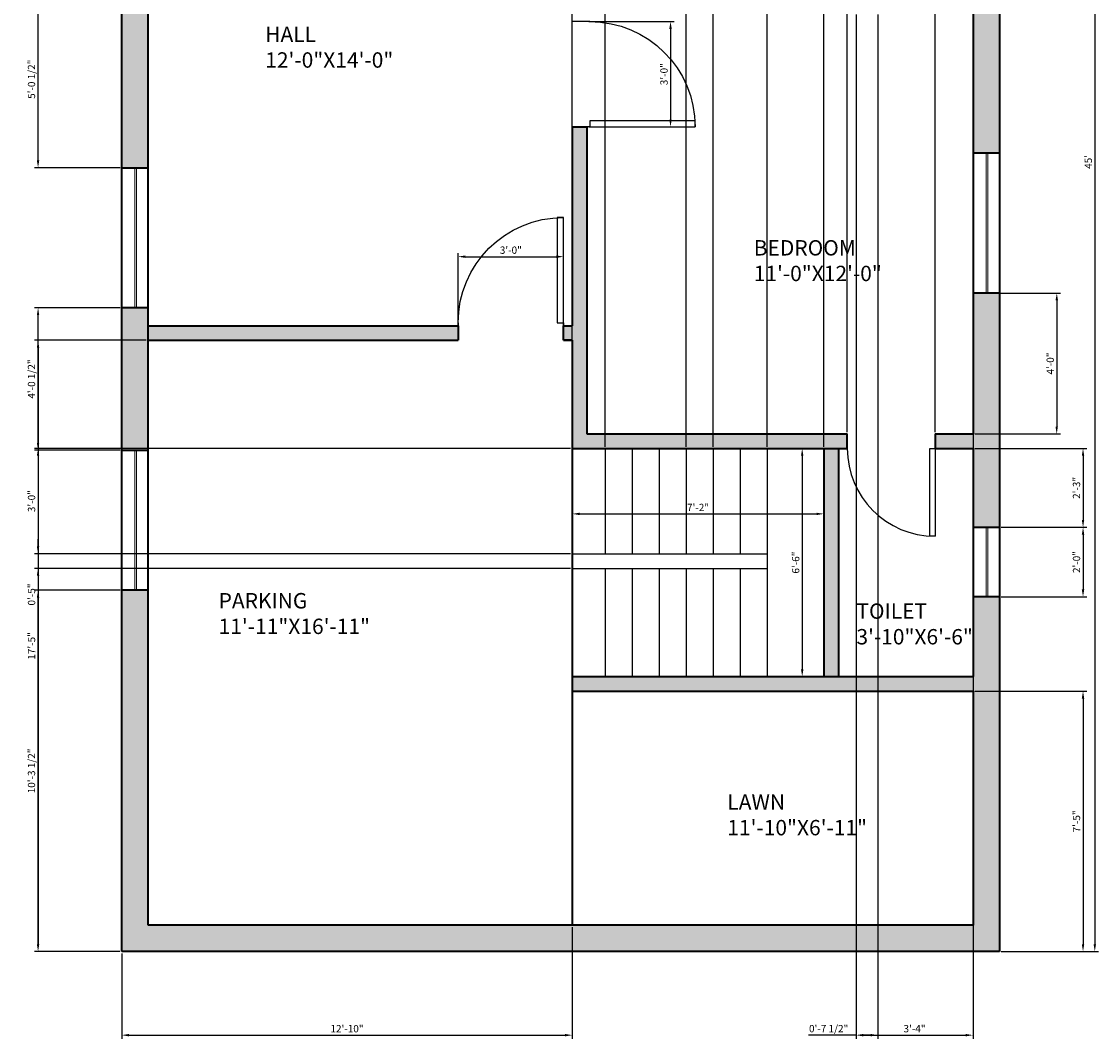
# Model space of a CAD drawing. Units: inches. Extents: x 2545 to 2915, y 1754 to 2359.
# Tile 1 of 2: x 2545 to 2913, y 1754 to 2103. Entities that reach past the tile are written whole.
import ezdxf

# ---------------------------------------------------------------- set-up
doc = ezdxf.new("R2010")
doc.units = ezdxf.units.IN
for name, color, linetype, lineweight in [('A-ANNO-DIMS', 2, 'Continuous', 18), ('A-AREA-IDEN', 7, 'Continuous', 25), ('A-DOOR', 3, 'Continuous', 25), ('A-FLOR-STRS', 7, 'Continuous', 25), ('A-GLAZ', 4, 'Continuous', 18), ('A-WALL', 7, 'Continuous', 35), ('A-WALL-PATT', 252, 'Continuous', 13)]:
    doc.layers.add(name, color=color, linetype=linetype, lineweight=lineweight)
doc.styles.get("Standard").update_dxf_attribs({"font": 'arial.ttf'})
doc.dimstyles.new('ISO-25', dxfattribs={"dimtxt": 2.5, "dimasz": 2.5, "dimexe": 1.25, "dimexo": 0.625, "dimtad": 1, "dimlunit": 4, "dimtxsty": 'Standard', "dimcen": 2.5, "dimadec": 0, "dimazin": 0, "dimtfac": 1, "dimtmove": 0, "dimatfit": 3, "dimfxl": 1, "dimarcsym": 0})

# ---------------------------------------------------------------- blocks, each defined once
blk = doc.blocks.new('*U2')
for p, q in [((0, 0), (0, -5)), ((30, 0), (30, -5))]:
    blk.add_line(p, q)
blk.add_lwpolyline([(0, 0), (0, 30), (1.75, 30), (1.75, 0)], close=True)
blk.add_arc((0, 0), 30, 0, 90)
blk = doc.blocks.new('*D4')
at = {"layer": 'A-ANNO-DIMS', "color": 0, "lineweight": -2, "transparency": 16777216}
for p, q in [((2880.02, 2324.74), (2913.27, 2324.74)), ((2912.02, 2322.24), (2912.02, 1787.24)), ((2880.02, 1784.74), (2913.27, 1784.74))]:
    blk.add_line(p, q, dxfattribs=at)
at = {"layer": 'A-ANNO-DIMS', "color": 0, "transparency": 16777216}
for points in [[(2911.6, 2322.24), (2912.44, 2322.24), (2912.02, 2324.74)], [(2911.6, 1787.24), (2912.44, 1787.24), (2912.02, 1784.74)]]:
    blk.add_solid(points, dxfattribs=at)
at = {"layer": 'Defpoints', "color": 0, "transparency": 16777216}
for p in [(2879.4, 2324.74), (2879.4, 1784.74), (2912.02, 1784.74)]:
    blk.add_point(p, dxfattribs=at)
at = {"layer": 'A-ANNO-DIMS', "color": 0, "transparency": 16777216, "insert": (2910.12, 2054.74), "char_height": 2.5, "attachment_point": 5, "rotation": 90}
blk.add_mtext("45'", dxfattribs=at)
blk = doc.blocks.new('*D5')
at = {"layer": 'A-ANNO-DIMS', "color": 0, "lineweight": -2, "transparency": 16777216}
for p, q in [((2809.58, 1956.74), (2813.25, 1956.74)), ((2812, 1954.24), (2812, 1881.24)), ((2809.58, 1878.74), (2813.25, 1878.74))]:
    blk.add_line(p, q, dxfattribs=at)
at = {"layer": 'A-ANNO-DIMS', "color": 0, "transparency": 16777216}
for points in [[(2811.59, 1954.24), (2812.42, 1954.24), (2812, 1956.74)], [(2811.59, 1881.24), (2812.42, 1881.24), (2812, 1878.74)]]:
    blk.add_solid(points, dxfattribs=at)
at = {"layer": 'Defpoints', "color": 0, "transparency": 16777216}
for p in [(2808.96, 1956.74), (2808.96, 1878.74), (2812, 1878.74)]:
    blk.add_point(p, dxfattribs=at)
at = {"layer": 'A-ANNO-DIMS', "color": 0, "transparency": 16777216, "insert": (2810.1, 1917.74), "char_height": 2.5, "attachment_point": 5, "rotation": 90}
blk.add_mtext('6\'-6"', dxfattribs=at)
blk = doc.blocks.new('*D6')
at = {"layer": 'A-ANNO-DIMS', "color": 0, "lineweight": -2, "transparency": 16777216}
for p, q in [((2733.4, 1931.78), (2733.4, 1935.64)), ((2735.9, 1934.39), (2816.9, 1934.39)), ((2819.4, 1931.78), (2819.4, 1935.64))]:
    blk.add_line(p, q, dxfattribs=at)
at = {"layer": 'A-ANNO-DIMS', "color": 0, "transparency": 16777216}
for points in [[(2735.9, 1934.8), (2735.9, 1933.97), (2733.4, 1934.39)], [(2816.9, 1934.8), (2816.9, 1933.97), (2819.4, 1934.39)]]:
    blk.add_solid(points, dxfattribs=at)
at = {"layer": 'Defpoints', "color": 0, "transparency": 16777216}
for p in [(2819.4, 1934.39), (2733.4, 1931.15), (2819.4, 1931.15)]:
    blk.add_point(p, dxfattribs=at)
at = {"layer": 'A-ANNO-DIMS', "color": 0, "transparency": 16777216, "insert": (2776.4, 1936.27), "char_height": 2.5, "attachment_point": 5}
blk.add_mtext('7\'-2"', dxfattribs=at)
blk = doc.blocks.new('WIN-SASH-48')
for p, q in [((0, 8.97), (47.9, 8.97)), ((0, 4.48), (47.9, 4.48)), ((0, 3.98), (47.9, 3.98)), ((47.9, 0), (0, 0))]:
    blk.add_line(p, q)
blk = doc.blocks.new('*D13')
at = {"layer": 'A-ANNO-DIMS', "color": 0, "lineweight": -2, "transparency": 16777216}
for p, q in [((2578.81, 1908.27), (2549.55, 1908.27)), ((2550.8, 1787.24), (2550.8, 1905.77)), ((2578.77, 1784.74), (2549.55, 1784.74))]:
    blk.add_line(p, q, dxfattribs=at)
at = {"layer": 'A-ANNO-DIMS', "color": 0, "transparency": 16777216}
for points in [[(2550.38, 1905.77), (2551.21, 1905.77), (2550.8, 1908.27)], [(2550.38, 1787.24), (2551.21, 1787.24), (2550.8, 1784.74)]]:
    blk.add_solid(points, dxfattribs=at)
at = {"layer": 'Defpoints', "color": 0, "transparency": 16777216}
for p in [(2550.8, 1908.27), (2579.43, 1908.27), (2579.4, 1784.74)]:
    blk.add_point(p, dxfattribs=at)
at = {"layer": 'A-ANNO-DIMS', "color": 0, "transparency": 16777216, "insert": (2548.88, 1846.5), "char_height": 2.5, "attachment_point": 5, "rotation": 90}
blk.add_mtext('10\'-3 1/2"', dxfattribs=at)
blk = doc.blocks.new('*D14')
at = {"layer": 'A-ANNO-DIMS', "color": 0, "lineweight": -2, "transparency": 16777216}
for p, q in [((2578.81, 2004.84), (2549.55, 2004.84)), ((2550.8, 1958.67), (2550.8, 2002.34)), ((2578.81, 1956.17), (2549.55, 1956.17))]:
    blk.add_line(p, q, dxfattribs=at)
at = {"layer": 'A-ANNO-DIMS', "color": 0, "transparency": 16777216}
for points in [[(2550.38, 2002.34), (2551.21, 2002.34), (2550.8, 2004.84)], [(2550.38, 1958.67), (2551.21, 1958.67), (2550.8, 1956.17)]]:
    blk.add_solid(points, dxfattribs=at)
at = {"layer": 'Defpoints', "color": 0, "transparency": 16777216}
for p in [(2550.8, 2004.84), (2579.43, 2004.84), (2579.43, 1956.17)]:
    blk.add_point(p, dxfattribs=at)
at = {"layer": 'A-ANNO-DIMS', "color": 0, "transparency": 16777216, "insert": (2548.88, 1980.5), "char_height": 2.5, "attachment_point": 5, "rotation": 90}
blk.add_mtext('4\'-0 1/2"', dxfattribs=at)
blk = doc.blocks.new('*D15')
at = {"layer": 'A-ANNO-DIMS', "color": 0, "lineweight": -2, "transparency": 16777216}
for p, q in [((2578.81, 2113.29), (2549.55, 2113.29)), ((2550.8, 2055.24), (2550.8, 2110.79)), ((2578.81, 2052.74), (2549.55, 2052.74))]:
    blk.add_line(p, q, dxfattribs=at)
at = {"layer": 'A-ANNO-DIMS', "color": 0, "transparency": 16777216}
for points in [[(2550.38, 2110.79), (2551.21, 2110.79), (2550.8, 2113.29)], [(2550.38, 2055.24), (2551.21, 2055.24), (2550.8, 2052.74)]]:
    blk.add_solid(points, dxfattribs=at)
at = {"layer": 'Defpoints', "color": 0, "transparency": 16777216}
for p in [(2550.8, 2113.29), (2579.43, 2113.29), (2579.43, 2052.74)]:
    blk.add_point(p, dxfattribs=at)
at = {"layer": 'A-ANNO-DIMS', "color": 0, "transparency": 16777216, "insert": (2548.88, 2083.01), "char_height": 2.5, "attachment_point": 5, "rotation": 90}
blk.add_mtext('5\'-0 1/2"', dxfattribs=at)
blk = doc.blocks.new('*D18')
at = {"layer": 'A-ANNO-DIMS', "color": 0, "lineweight": -2, "transparency": 16777216}
for p, q in [((2871.06, 2009.91), (2900.28, 2009.88)), ((2899.03, 2007.39), (2899, 1964.22)), ((2871.02, 1961.74), (2900.25, 1961.72))]:
    blk.add_line(p, q, dxfattribs=at)
at = {"layer": 'A-ANNO-DIMS', "color": 0, "transparency": 16777216}
for points in [[(2898.61, 2007.39), (2899.45, 2007.39), (2899.03, 2009.89)], [(2898.58, 1964.22), (2899.41, 1964.22), (2899, 1961.72)]]:
    blk.add_solid(points, dxfattribs=at)
at = {"layer": 'Defpoints', "color": 0, "transparency": 16777216}
for p in [(2870.43, 2009.91), (2870.4, 1961.74), (2899, 1961.72)]:
    blk.add_point(p, dxfattribs=at)
at = {"layer": 'A-ANNO-DIMS', "color": 0, "transparency": 16777216, "insert": (2897.11, 1985.8), "char_height": 2.5, "attachment_point": 5, "rotation": 89.9593}
blk.add_mtext('4\'-0"', dxfattribs=at)
blk = doc.blocks.new('*D21')
at = {"layer": 'A-ANNO-DIMS', "color": 0, "lineweight": -2, "transparency": 16777216}
for p, q in [((2694.4, 1994.37), (2694.4, 2023.59)), ((2696.9, 2022.34), (2727.9, 2022.34)), ((2730.4, 1994.37), (2730.4, 2023.59))]:
    blk.add_line(p, q, dxfattribs=at)
at = {"layer": 'A-ANNO-DIMS', "color": 0, "transparency": 16777216}
for points in [[(2696.9, 2022.76), (2696.9, 2021.92), (2694.4, 2022.34)], [(2727.9, 2022.76), (2727.9, 2021.92), (2730.4, 2022.34)]]:
    blk.add_solid(points, dxfattribs=at)
at = {"layer": 'Defpoints', "color": 0, "transparency": 16777216}
for p in [(2730.4, 2022.34), (2694.4, 1993.74), (2730.4, 1993.74)]:
    blk.add_point(p, dxfattribs=at)
at = {"layer": 'A-ANNO-DIMS', "color": 0, "transparency": 16777216, "insert": (2712.4, 2024.24), "char_height": 2.5, "attachment_point": 5}
blk.add_mtext('3\'-0"', dxfattribs=at)
blk = doc.blocks.new('*D24')
at = {"layer": 'A-ANNO-DIMS', "color": 0, "lineweight": -2, "transparency": 16777216}
for p, q in [((2739.02, 2102.74), (2768.25, 2102.74)), ((2767, 2100.24), (2767, 2069.24)), ((2739.02, 2066.74), (2768.25, 2066.74))]:
    blk.add_line(p, q, dxfattribs=at)
at = {"layer": 'A-ANNO-DIMS', "color": 0, "transparency": 16777216}
for points in [[(2766.58, 2100.24), (2767.41, 2100.24), (2767, 2102.74)], [(2766.58, 2069.24), (2767.41, 2069.24), (2767, 2066.74)]]:
    blk.add_solid(points, dxfattribs=at)
at = {"layer": 'Defpoints', "color": 0, "transparency": 16777216}
for p in [(2738.4, 2102.74), (2738.4, 2066.74), (2767, 2066.74)]:
    blk.add_point(p, dxfattribs=at)
at = {"layer": 'A-ANNO-DIMS', "color": 0, "transparency": 16777216, "insert": (2765.09, 2084.74), "char_height": 2.5, "attachment_point": 5, "rotation": 90}
blk.add_mtext('3\'-0"', dxfattribs=at)
blk = doc.blocks.new('*D26')
at = {"layer": 'A-ANNO-DIMS', "color": 0, "lineweight": -2, "transparency": 16777216}
for p, q in [((2733.4, 1793.12), (2733.4, 1754.89)), ((2579.4, 1784.12), (2579.4, 1754.89)), ((2581.9, 1756.14), (2730.9, 1756.14))]:
    blk.add_line(p, q, dxfattribs=at)
at = {"layer": 'A-ANNO-DIMS', "color": 0, "transparency": 16777216}
for points in [[(2581.9, 1756.56), (2581.9, 1755.72), (2579.4, 1756.14)], [(2730.9, 1756.56), (2730.9, 1755.72), (2733.4, 1756.14)]]:
    blk.add_solid(points, dxfattribs=at)
at = {"layer": 'Defpoints', "color": 0, "transparency": 16777216}
for p in [(2733.4, 1793.74), (2579.4, 1784.74), (2733.4, 1756.14)]:
    blk.add_point(p, dxfattribs=at)
at = {"layer": 'A-ANNO-DIMS', "color": 0, "transparency": 16777216, "insert": (2656.4, 1758.04), "char_height": 2.5, "attachment_point": 5}
blk.add_mtext('12\'-10"', dxfattribs=at)
blk = doc.blocks.new('*D27')
at = {"layer": 'A-ANNO-DIMS', "color": 0, "lineweight": -2, "transparency": 16777216}
for p, q in [((2587.77, 1993.74), (2549.55, 1993.74)), ((2550.8, 1991.24), (2550.8, 1787.24)), ((2578.77, 1784.74), (2549.55, 1784.74))]:
    blk.add_line(p, q, dxfattribs=at)
at = {"layer": 'A-ANNO-DIMS', "color": 0, "transparency": 16777216}
for points in [[(2550.38, 1991.24), (2551.21, 1991.24), (2550.8, 1993.74)], [(2550.38, 1787.24), (2551.21, 1787.24), (2550.8, 1784.74)]]:
    blk.add_solid(points, dxfattribs=at)
at = {"layer": 'Defpoints', "color": 0, "transparency": 16777216}
for p in [(2588.4, 1993.74), (2550.8, 1784.74), (2579.4, 1784.74)]:
    blk.add_point(p, dxfattribs=at)
at = {"layer": 'A-ANNO-DIMS', "color": 0, "transparency": 16777216, "insert": (2548.89, 1889.24), "char_height": 2.5, "attachment_point": 5, "rotation": 90}
blk.add_mtext('17\'-5"', dxfattribs=at)
blk = doc.blocks.new('*D28')
at = {"layer": 'A-ANNO-DIMS', "color": 0, "lineweight": -2, "transparency": 16777216}
for p, q in [((2871.02, 1873.74), (2909.25, 1873.74)), ((2908, 1871.24), (2908, 1787.24)), ((2880.02, 1784.74), (2909.25, 1784.74))]:
    blk.add_line(p, q, dxfattribs=at)
at = {"layer": 'A-ANNO-DIMS', "color": 0, "transparency": 16777216}
for points in [[(2907.58, 1871.24), (2908.41, 1871.24), (2908, 1873.74)], [(2907.58, 1787.24), (2908.41, 1787.24), (2908, 1784.74)]]:
    blk.add_solid(points, dxfattribs=at)
at = {"layer": 'Defpoints', "color": 0, "transparency": 16777216}
for p in [(2870.4, 1873.74), (2879.4, 1784.74), (2908, 1784.74)]:
    blk.add_point(p, dxfattribs=at)
at = {"layer": 'A-ANNO-DIMS', "color": 0, "transparency": 16777216, "insert": (2906.1, 1829.24), "char_height": 2.5, "attachment_point": 5, "rotation": 90}
blk.add_mtext('7\'-5"', dxfattribs=at)
blk = doc.blocks.new('*D29')
at = {"layer": 'A-ANNO-DIMS', "color": 0, "lineweight": -2, "transparency": 16777216}
for p, q in [((2827.4, 1962.37), (2827.4, 2354.59)), ((2829.9, 2353.34), (2854.9, 2353.34)), ((2857.4, 1962.37), (2857.4, 2354.59))]:
    blk.add_line(p, q, dxfattribs=at)
at = {"layer": 'A-ANNO-DIMS', "color": 0, "transparency": 16777216}
for points in [[(2829.9, 2353.76), (2829.9, 2352.92), (2827.4, 2353.34)], [(2854.9, 2353.76), (2854.9, 2352.92), (2857.4, 2353.34)]]:
    blk.add_solid(points, dxfattribs=at)
at = {"layer": 'Defpoints', "color": 0, "transparency": 16777216}
for p in [(2857.4, 2353.34), (2827.4, 1961.74), (2857.4, 1961.74)]:
    blk.add_point(p, dxfattribs=at)
at = {"layer": 'A-ANNO-DIMS', "color": 0, "transparency": 16777216, "insert": (2842.4, 2355.24), "char_height": 2.5, "attachment_point": 5}
blk.add_mtext('2\'-6"', dxfattribs=at)
blk = doc.blocks.new('*D30')
at = {"layer": 'A-ANNO-DIMS', "color": 0, "lineweight": -2, "transparency": 16777216}
for p, q in [((2857.4, 1962.37), (2857.4, 2354.59)), ((2859.9, 2353.34), (2867.9, 2353.34)), ((2870.4, 1962.37), (2870.4, 2354.59))]:
    blk.add_line(p, q, dxfattribs=at)
at = {"layer": 'A-ANNO-DIMS', "color": 0, "transparency": 16777216}
for points in [[(2859.9, 2353.76), (2859.9, 2352.92), (2857.4, 2353.34)], [(2867.9, 2353.76), (2867.9, 2352.92), (2870.4, 2353.34)]]:
    blk.add_solid(points, dxfattribs=at)
at = {"layer": 'Defpoints', "color": 0, "transparency": 16777216}
for p in [(2870.4, 2353.34), (2857.4, 1961.74), (2870.4, 1961.74)]:
    blk.add_point(p, dxfattribs=at)
at = {"layer": 'A-ANNO-DIMS', "color": 0, "transparency": 16777216, "insert": (2863.9, 2355.22), "char_height": 2.5, "attachment_point": 5}
blk.add_mtext('1\'-1"', dxfattribs=at)
blk = doc.blocks.new('*D31')
at = {"layer": 'A-ANNO-DIMS', "color": 0, "lineweight": -2, "transparency": 16777216}
for p, q in [((2772.31, 1957.37), (2772.31, 2354.59)), ((2774.81, 2353.34), (2779.04, 2353.34)), ((2781.54, 1957.37), (2781.54, 2354.59))]:
    blk.add_line(p, q, dxfattribs=at)
at = {"layer": 'A-ANNO-DIMS', "color": 0, "transparency": 16777216}
for points in [[(2774.81, 2353.76), (2774.81, 2352.92), (2772.31, 2353.34)], [(2779.04, 2353.76), (2779.04, 2352.92), (2781.54, 2353.34)]]:
    blk.add_solid(points, dxfattribs=at)
at = {"layer": 'Defpoints', "color": 0, "transparency": 16777216}
for p in [(2781.54, 2353.34), (2772.31, 1956.74), (2781.54, 1956.74)]:
    blk.add_point(p, dxfattribs=at)
at = {"layer": 'A-ANNO-DIMS', "color": 0, "transparency": 16777216, "insert": (2776.92, 2355.24), "char_height": 2.5, "attachment_point": 5}
blk.add_mtext('0\'-9"', dxfattribs=at)
blk = doc.blocks.new('*D32')
at = {"layer": 'A-ANNO-DIMS', "color": 0, "lineweight": -2, "transparency": 16777216}
for p, q in [((2800, 1957.37), (2800, 2354.59)), ((2802.5, 2353.34), (2816.9, 2353.34)), ((2819.4, 1957.37), (2819.4, 2354.59))]:
    blk.add_line(p, q, dxfattribs=at)
at = {"layer": 'A-ANNO-DIMS', "color": 0, "transparency": 16777216}
for points in [[(2802.5, 2353.76), (2802.5, 2352.92), (2800, 2353.34)], [(2816.9, 2353.76), (2816.9, 2352.92), (2819.4, 2353.34)]]:
    blk.add_solid(points, dxfattribs=at)
at = {"layer": 'Defpoints', "color": 0, "transparency": 16777216}
for p in [(2819.4, 2353.34), (2800, 1956.74), (2819.4, 1956.74)]:
    blk.add_point(p, dxfattribs=at)
at = {"layer": 'A-ANNO-DIMS', "color": 0, "transparency": 16777216, "insert": (2809.7, 2355.26), "char_height": 2.5, "attachment_point": 5}
blk.add_mtext('1\'-7 1/2"', dxfattribs=at)
blk = doc.blocks.new('*D33')
at = {"layer": 'A-ANNO-DIMS', "color": 0, "lineweight": -2, "transparency": 16777216}
for p, q in [((2732.77, 1956.74), (2549.55, 1956.74)), ((2550.8, 1954.24), (2550.8, 1923.27)), ((2732.77, 1920.77), (2549.55, 1920.77))]:
    blk.add_line(p, q, dxfattribs=at)
at = {"layer": 'A-ANNO-DIMS', "color": 0, "transparency": 16777216}
for points in [[(2550.38, 1954.24), (2551.21, 1954.24), (2550.8, 1956.74)], [(2550.38, 1923.27), (2551.21, 1923.27), (2550.8, 1920.77)]]:
    blk.add_solid(points, dxfattribs=at)
at = {"layer": 'Defpoints', "color": 0, "transparency": 16777216}
for p in [(2733.4, 1956.74), (2550.8, 1920.77), (2733.4, 1920.77)]:
    blk.add_point(p, dxfattribs=at)
at = {"layer": 'A-ANNO-DIMS', "color": 0, "transparency": 16777216, "insert": (2548.89, 1938.75), "char_height": 2.5, "attachment_point": 5, "rotation": 90}
blk.add_mtext('3\'-0"', dxfattribs=at)
blk = doc.blocks.new('*D34')
at = {"layer": 'A-ANNO-DIMS', "color": 0, "lineweight": -2, "transparency": 16777216}
for p, q in [((2550.8, 1923.27), (2550.8, 1925.77)), ((2732.77, 1920.77), (2549.55, 1920.77)), ((2550.8, 1920.77), (2550.8, 1915.77)), ((2732.77, 1915.77), (2549.55, 1915.77)), ((2550.8, 1913.27), (2550.8, 1902.87))]:
    blk.add_line(p, q, dxfattribs=at)
at = {"layer": 'A-ANNO-DIMS', "color": 0, "transparency": 16777216}
for points in [[(2550.38, 1923.27), (2551.21, 1923.27), (2550.8, 1920.77)], [(2550.38, 1913.27), (2551.21, 1913.27), (2550.8, 1915.77)]]:
    blk.add_solid(points, dxfattribs=at)
at = {"layer": 'Defpoints', "color": 0, "transparency": 16777216}
for p in [(2733.4, 1920.77), (2550.8, 1915.77), (2733.4, 1915.77)]:
    blk.add_point(p, dxfattribs=at)
at = {"layer": 'A-ANNO-DIMS', "color": 0, "transparency": 16777216, "insert": (2548.89, 1906.82), "char_height": 2.5, "attachment_point": 5, "rotation": 90}
blk.add_mtext('0\'-5"', dxfattribs=at)
blk = doc.blocks.new('*D35')
at = {"layer": 'A-ANNO-DIMS', "color": 0, "lineweight": -2, "transparency": 16777216}
for p, q in [((2733.4, 1957.37), (2733.4, 2354.59)), ((2735.9, 2353.34), (2742.11, 2353.34)), ((2744.61, 1957.37), (2744.61, 2354.59))]:
    blk.add_line(p, q, dxfattribs=at)
at = {"layer": 'A-ANNO-DIMS', "color": 0, "transparency": 16777216}
for points in [[(2735.9, 2353.76), (2735.9, 2352.92), (2733.4, 2353.34)], [(2742.11, 2353.76), (2742.11, 2352.92), (2744.61, 2353.34)]]:
    blk.add_solid(points, dxfattribs=at)
at = {"layer": 'Defpoints', "color": 0, "transparency": 16777216}
for p in [(2744.61, 2353.34), (2733.4, 1956.74), (2744.61, 1956.74)]:
    blk.add_point(p, dxfattribs=at)
at = {"layer": 'A-ANNO-DIMS', "color": 0, "transparency": 16777216, "insert": (2739.01, 2355.24), "char_height": 2.5, "attachment_point": 5}
blk.add_mtext('0\'-11"', dxfattribs=at)
blk = doc.blocks.new('*D36')
at = {"layer": 'A-ANNO-DIMS', "color": 0, "lineweight": -2, "transparency": 16777216}
for p, q in [((2880.02, 1929.8), (2909.25, 1929.8)), ((2908, 1927.3), (2908, 1908.54)), ((2880.02, 1906.04), (2909.25, 1906.04))]:
    blk.add_line(p, q, dxfattribs=at)
at = {"layer": 'A-ANNO-DIMS', "color": 0, "transparency": 16777216}
for points in [[(2907.58, 1927.3), (2908.41, 1927.3), (2908, 1929.8)], [(2907.58, 1908.54), (2908.41, 1908.54), (2908, 1906.04)]]:
    blk.add_solid(points, dxfattribs=at)
at = {"layer": 'Defpoints', "color": 0, "transparency": 16777216}
for p in [(2879.4, 1929.8), (2879.4, 1906.04), (2908, 1906.04)]:
    blk.add_point(p, dxfattribs=at)
at = {"layer": 'A-ANNO-DIMS', "color": 0, "transparency": 16777216, "insert": (2906.09, 1917.92), "char_height": 2.5, "attachment_point": 5, "rotation": 90}
blk.add_mtext('2\'-0"', dxfattribs=at)
blk = doc.blocks.new('*D37')
at = {"layer": 'A-ANNO-DIMS', "color": 0, "lineweight": -2, "transparency": 16777216}
for p, q in [((2871.02, 1956.74), (2909.25, 1956.74)), ((2908, 1954.24), (2908, 1932.3)), ((2880.02, 1929.8), (2909.25, 1929.8))]:
    blk.add_line(p, q, dxfattribs=at)
at = {"layer": 'A-ANNO-DIMS', "color": 0, "transparency": 16777216}
for points in [[(2907.58, 1954.24), (2908.41, 1954.24), (2908, 1956.74)], [(2907.58, 1932.3), (2908.41, 1932.3), (2908, 1929.8)]]:
    blk.add_solid(points, dxfattribs=at)
at = {"layer": 'Defpoints', "color": 0, "transparency": 16777216}
for p in [(2870.4, 1956.74), (2879.4, 1929.8), (2908, 1929.8)]:
    blk.add_point(p, dxfattribs=at)
at = {"layer": 'A-ANNO-DIMS', "color": 0, "transparency": 16777216, "insert": (2906.09, 1943.27), "char_height": 2.5, "attachment_point": 5, "rotation": 90}
blk.add_mtext('2\'-3"', dxfattribs=at)
blk = doc.blocks.new('*D41')
at = {"layer": 'A-ANNO-DIMS', "color": 0, "lineweight": -2, "transparency": 16777216}
for p, q in [((2830.4, 2105.12), (2830.4, 1754.89)), ((2837.91, 2105.12), (2837.91, 1754.89)), ((2830.4, 1756.14), (2814.17, 1756.14)), ((2835.41, 1756.14), (2832.9, 1756.14))]:
    blk.add_line(p, q, dxfattribs=at)
at = {"layer": 'A-ANNO-DIMS', "color": 0, "transparency": 16777216}
for points in [[(2832.9, 1756.56), (2832.9, 1755.72), (2830.4, 1756.14)], [(2835.41, 1756.56), (2835.41, 1755.72), (2837.91, 1756.14)]]:
    blk.add_solid(points, dxfattribs=at)
at = {"layer": 'Defpoints', "color": 0, "transparency": 16777216}
for p in [(2830.4, 2105.74), (2837.91, 2105.74), (2830.4, 1756.14)]:
    blk.add_point(p, dxfattribs=at)
at = {"layer": 'A-ANNO-DIMS', "color": 0, "transparency": 16777216, "insert": (2821.04, 1758.06), "char_height": 2.5, "attachment_point": 5}
blk.add_mtext('0\'-7 1/2"', dxfattribs=at)
blk = doc.blocks.new('*D43')
at = {"layer": 'A-ANNO-DIMS', "color": 0, "lineweight": -2, "transparency": 16777216}
for p, q in [((2830.4, 2105.12), (2830.4, 1754.89)), ((2870.4, 2105.12), (2870.4, 1754.89)), ((2832.9, 1756.14), (2867.9, 1756.14))]:
    blk.add_line(p, q, dxfattribs=at)
at = {"layer": 'A-ANNO-DIMS', "color": 0, "transparency": 16777216}
for points in [[(2832.9, 1756.56), (2832.9, 1755.72), (2830.4, 1756.14)], [(2867.9, 1756.56), (2867.9, 1755.72), (2870.4, 1756.14)]]:
    blk.add_solid(points, dxfattribs=at)
at = {"layer": 'Defpoints', "color": 0, "transparency": 16777216}
for p in [(2830.4, 2105.74), (2870.4, 2105.74), (2870.4, 1756.14)]:
    blk.add_point(p, dxfattribs=at)
at = {"layer": 'A-ANNO-DIMS', "color": 0, "transparency": 16777216, "insert": (2850.4, 1758.04), "char_height": 2.5, "attachment_point": 5}
blk.add_mtext('3\'-4"', dxfattribs=at)

msp = doc.modelspace()

# ---------------------------------------------------------------- hatches: boundary and pattern name
at = {"layer": 'A-WALL-PATT'}
h = msp.add_hatch(color=256, dxfattribs=at)
h.dxf.hatch_style = 1
h.paths.add_polyline_path([(2879.396, 2222.429), (2870.396, 2222.429), (2870.396, 2171.741), (2862.945, 2171.741), (2862.945, 2166.741), (2870.396, 2166.741), (2870.396, 2110.741), (2864.62, 2110.741), (2864.62, 2105.741), (2870.396, 2105.741), (2870.396, 2057.805), (2879.396, 2057.805)])
h = msp.add_hatch(color=256, dxfattribs=at)
h.dxf.hatch_style = 1
h.paths.add_polyline_path([(2588.396, 2113.285), (2579.396, 2113.285), (2579.396, 2052.737), (2588.396, 2052.737)])
h = msp.add_hatch(color=256, dxfattribs=at)
h.dxf.hatch_style = 1
h.paths.add_polyline_path([(2827.396, 1961.741), (2738.396, 1961.741), (2738.396, 2066.741), (2733.396, 2066.741), (2733.396, 1998.741), (2730.396, 1998.741), (2730.396, 1993.741), (2733.396, 1993.741), (2733.396, 1956.741), (2827.396, 1956.741)])
h = msp.add_hatch(color=256, dxfattribs=at)
h.dxf.hatch_style = 1
h.paths.add_polyline_path([(2879.396, 2009.906), (2870.396, 2009.906), (2870.396, 1961.741), (2857.396, 1961.741), (2857.396, 1956.741), (2870.396, 1956.741), (2870.396, 1929.796), (2879.396, 1929.796)])
h = msp.add_hatch(color=256, dxfattribs=at)
h.dxf.hatch_style = 1
h.paths.add_polyline_path([(2588.396, 2004.839), (2579.396, 2004.839), (2579.396, 1956.168), (2588.396, 1956.168)])
h = msp.add_hatch(color=256, dxfattribs=at)
h.dxf.hatch_style = 1
h.paths.add_polyline_path([(2694.396, 1998.741), (2588.396, 1998.741), (2588.396, 1993.741), (2694.396, 1993.741)])
h = msp.add_hatch(color=256, dxfattribs=at)
h.dxf.hatch_style = 1
h.paths.add_polyline_path([(2824.396, 1956.741), (2819.396, 1956.741), (2819.396, 1878.741), (2824.396, 1878.741)])
h = msp.add_hatch(color=256, dxfattribs=at)
h.dxf.hatch_style = 1
h.paths.add_polyline_path([(2879.396, 1906.044), (2870.396, 1906.044), (2870.396, 1878.741), (2733.396, 1878.741), (2733.396, 1873.741), (2870.396, 1873.741), (2870.396, 1793.741), (2588.396, 1793.741), (2588.396, 1908.269), (2579.396, 1908.269), (2579.396, 1784.741), (2879.396, 1784.741)])
h.paths.add_polyline_path([(2828.912, 1886.761), (2869.796, 1886.761), (2869.796, 1906.39), (2828.912, 1906.39)], flags=25)

# ---------------------------------------------------------------- linework, layer by layer
at = {"layer": 'A-FLOR-STRS'}
for p, q in [((2744.614, 1956.741), (2744.614, 1920.767)), ((2753.845, 1956.741), (2753.845, 1920.767)), ((2763.075, 1956.741), (2763.075, 1920.767)), ((2772.305, 1956.741), (2772.305, 1920.767)), ((2781.535, 1956.741), (2781.535, 1920.767)), ((2790.766, 1956.741), (2790.766, 1920.767)), ((2799.996, 1956.741), (2799.996, 1878.741)), ((2733.396, 1920.767), (2799.996, 1920.767)), ((2733.396, 1915.767), (2799.996, 1915.767)), ((2744.614, 1915.767), (2744.614, 1878.741)), ((2753.845, 1915.767), (2753.845, 1878.741)), ((2763.075, 1915.767), (2763.075, 1878.741)), ((2772.305, 1915.767), (2772.305, 1878.741)), ((2781.535, 1915.767), (2781.535, 1878.741)), ((2790.766, 1915.767), (2790.766, 1878.741))]:
    msp.add_line(p, q, dxfattribs=at)
at = {"layer": 'A-GLAZ'}
for p, q in [((2870.485, 1906.044), (2870.485, 1929.796)), ((2874.941, 1906.044), (2874.941, 1929.796)), ((2875.438, 1906.044), (2875.438, 1929.796)), ((2879.396, 1929.796), (2879.396, 1906.044))]:
    msp.add_line(p, q, dxfattribs=at)
at = {"layer": 'A-WALL'}
for p, q in [((2579.396, 1784.741), (2579.396, 2324.741)), ((2879.396, 2324.741), (2879.396, 1784.741)), ((2588.396, 1793.741), (2588.396, 2319.741)), ((2870.396, 2105.741), (2870.396, 1961.741)), ((2733.396, 2066.741), (2738.396, 2066.741)), ((2733.396, 2066.741), (2733.396, 1998.741)), ((2738.396, 2066.741), (2738.396, 1961.741)), ((2870.43, 2057.805), (2879.396, 2057.805)), ((2579.43, 2052.737), (2588.396, 2052.737)), ((2879.396, 2009.906), (2870.43, 2009.906)), ((2588.396, 2004.839), (2579.43, 2004.839)), ((2588.396, 1998.741), (2694.396, 1998.741)), ((2694.396, 1998.741), (2694.396, 1993.741)), ((2730.396, 1993.741), (2730.396, 1998.741)), ((2730.396, 1998.741), (2733.396, 1998.741)), ((2588.396, 1993.741), (2694.396, 1993.741)), ((2733.396, 1993.741), (2730.396, 1993.741)), ((2730.396, 1993.741), (2733.396, 1993.741)), ((2733.396, 1993.741), (2733.396, 1793.741)), ((2738.396, 1961.741), (2827.396, 1961.741)), ((2827.396, 1956.741), (2827.396, 1961.741)), ((2857.396, 1961.741), (2857.396, 1956.741)), ((2857.396, 1961.741), (2870.396, 1961.741)), ((2579.43, 1956.168), (2588.396, 1956.168)), ((2733.396, 1956.741), (2827.396, 1956.741)), ((2819.396, 1956.741), (2819.396, 1878.741)), ((2824.396, 1956.741), (2824.396, 1878.741)), ((2824.396, 1956.741), (2827.396, 1956.741)), ((2857.396, 1956.741), (2870.396, 1956.741)), ((2870.396, 1956.741), (2870.396, 1878.741)), ((2870.485, 1929.796), (2879.396, 1929.796)), ((2588.396, 1908.269), (2579.43, 1908.269)), ((2879.396, 1906.044), (2870.485, 1906.044)), ((2733.396, 1878.741), (2870.396, 1878.741)), ((2733.396, 1873.741), (2870.396, 1873.741)), ((2870.396, 1873.741), (2870.396, 1793.741)), ((2870.396, 1793.741), (2588.396, 1793.741)), ((2879.396, 1784.741), (2579.396, 1784.741))]:
    msp.add_line(p, q, dxfattribs=at)

# ---------------------------------------------------------------- block references
at = {"layer": 'A-DOOR', "xscale": -1.199999999999999, "yscale": 1.199999999999999, "zscale": 1.199999999999999, "rotation": 270}
msp.add_blockref('*U2', (2739.396, 2066.741), dxfattribs=at)
at = {"layer": 'A-DOOR', "xscale": -1.199999999999999, "yscale": 1.199999999999999, "zscale": 1.199999999999999}
msp.add_blockref('*U2', (2730.396, 1999.741), dxfattribs=at)
at = {"layer": 'A-DOOR', "rotation": 180}
msp.add_blockref('*U2', (2857.396, 1956.741), dxfattribs=at)
at = {"layer": 'A-GLAZ'}
for p, rotation in [((2879.396, 2009.906), 90.00000000000179), ((2588.396, 2004.839), 90.00000000000087), ((2588.396, 1908.269), 90.00000000000095)]:
    msp.add_blockref('WIN-SASH-48', p, dxfattribs=dict(at, rotation=rotation))

# ---------------------------------------------------------------- texts
at = {"layer": 'A-AREA-IDEN', "char_height": 5.26031, "attachment_point": 1}
for s, insert in [('HALL\\P12\'-0"X14\'-0"', (2628.452, 2100.987)), ('BEDROOM\\P11\'-0"X12\'-0"', (2795.429, 2027.996)), ('PARKING\\P11\'-11"X16\'-11"', (2612.517, 1907.325)), ('TOILET\\P3\'-10"X6\'-6"', (2830.536, 1903.776)), ('LAWN\\P11\'-10"X6\'-11"', (2786.397, 1838.505))]:
    msp.add_mtext_dynamic_manual_height_columns(s, width=4.6518, gutter_width=26.302, heights=[0], dxfattribs=dict(at, insert=insert))

# ---------------------------------------------------------------- dimensions: what is measured, and where the dimension line sits
at = {"layer": 'A-ANNO-DIMS'}
for base, p1, p2, override, picture, middle in [((2744.614, 2353.341), (2733.396, 1956.741), (2744.614, 1956.741), {"dimdec": 1, "dimlfac": 1, "dimrnd": 0, "dimzin": 1, "dimdsep": 46, "dimlunit": 4, "dimfrac": 2}, '*D35', (2739.005, 2355.242)), ((2781.535, 2353.341), (2772.305, 1956.741), (2781.535, 1956.741), {"dimdec": 1, "dimlfac": 1, "dimrnd": 0, "dimzin": 1, "dimdsep": 46, "dimlunit": 4, "dimfrac": 2}, '*D31', (2776.92, 2355.242)), ((2819.396, 2353.341), (2799.996, 1956.741), (2819.396, 1956.741), {"dimdec": 1, "dimlfac": 1, "dimrnd": 0, "dimzin": 1, "dimdsep": 46, "dimlunit": 4, "dimfrac": 2}, '*D32', (2809.696, 2355.259)), ((2857.396, 2353.341), (2827.396, 1961.741), (2857.396, 1961.741), {"dimdec": 1, "dimlfac": 1, "dimrnd": 0, "dimzin": 1, "dimdsep": 46, "dimlunit": 4, "dimfrac": 2}, '*D29', (2842.396, 2355.242)), ((2870.396, 2353.341), (2857.396, 1961.741), (2870.396, 1961.741), {"dimdec": 1, "dimlfac": 1, "dimrnd": 0, "dimzin": 1, "dimdsep": 46, "dimlunit": 4, "dimfrac": 2}, '*D30', (2863.896, 2355.221)), ((2830.396, 1756.141), (2837.908, 2105.741), (2830.396, 2105.741), {"dimdec": 1, "dimlfac": 1, "dimrnd": 0, "dimzin": 1, "dimdsep": 46, "dimlunit": 4, "dimfrac": 2}, '*D41', (2821.035, 1758.059)), ((2870.396, 1756.141), (2830.396, 2105.741), (2870.396, 2105.741), {"dimdec": 1, "dimlfac": 1, "dimrnd": 0, "dimzin": 1, "dimdsep": 46, "dimlunit": 4, "dimfrac": 2}, '*D43', (2850.396, 1758.043)), ((2730.396, 2022.341), (2694.396, 1993.741), (2730.396, 1993.741), {"dimdec": 1, "dimlfac": 1, "dimrnd": 0, "dimzin": 1, "dimdsep": 46, "dimlunit": 4, "dimfrac": 2}, '*D21', (2712.396, 2024.243)), ((2819.396, 1934.387), (2733.396, 1931.152), (2819.396, 1931.152), {"dimclrd": 0, "dimclre": 0, "dimclrt": 0}, '*D6', (2776.396, 1936.267)), ((2733.396, 1756.141), (2579.396, 1784.741), (2733.396, 1793.741), {"dimdec": 1, "dimlfac": 1, "dimrnd": 0, "dimzin": 1, "dimdsep": 46, "dimlunit": 4, "dimfrac": 2}, '*D26', (2656.396, 1758.042))]:
    dim = msp.add_linear_dim(base=base, p1=p1, p2=p2, dimstyle='ISO-25', override=override, dxfattribs=at)
    dim.commit()
    dim.dimension.update_dxf_attribs({"geometry": picture, "text_midpoint": middle})
for base, p1, p2, angle, override, picture, middle in [((2912.021, 1784.741), (2879.396, 2324.741), (2879.396, 1784.741), 90, {"dimclrd": 0, "dimclre": 0, "dimclrt": 0}, '*D4', (2910.125, 2054.741)), ((2550.796, 2113.285), (2579.43, 2052.737), (2579.43, 2113.285), 90, {"dimdec": 1, "dimlfac": 1, "dimrnd": 0, "dimzin": 1, "dimdsep": 46, "dimlunit": 4, "dimfrac": 2}, '*D15', (2548.878, 2083.011)), ((2766.996, 2066.741), (2738.396, 2102.741), (2738.396, 2066.741), 270, {"dimdec": 1, "dimlfac": 1, "dimrnd": 0, "dimzin": 1, "dimdsep": 46, "dimlunit": 4, "dimfrac": 2}, '*D24', (2765.094, 2084.741)), ((2898.996, 1961.721), (2870.43, 2009.906), (2870.396, 1961.741), 269.9593, {"dimdec": 1, "dimlfac": 1, "dimrnd": 0, "dimzin": 1, "dimdsep": 46, "dimlunit": 4, "dimfrac": 2}, '*D18', (2897.112, 1985.804)), ((2550.796, 2004.839), (2579.43, 1956.168), (2579.43, 2004.839), 90, {"dimdec": 1, "dimlfac": 1, "dimrnd": 0, "dimzin": 1, "dimdsep": 46, "dimlunit": 4, "dimfrac": 2}, '*D14', (2548.878, 1980.503)), ((2550.796, 1784.741), (2588.396, 1993.741), (2579.396, 1784.741), 90, {"dimdec": 1, "dimlfac": 1, "dimrnd": 0, "dimzin": 1, "dimdsep": 46, "dimlunit": 4, "dimfrac": 2}, '*D27', (2548.894, 1889.241)), ((2550.796, 1920.767), (2733.396, 1956.741), (2733.396, 1920.767), 90, {"dimdec": 1, "dimlfac": 1, "dimrnd": 0, "dimzin": 1, "dimdsep": 46, "dimlunit": 4, "dimfrac": 2}, '*D33', (2548.894, 1938.754)), ((2812.002, 1878.741), (2808.955, 1956.741), (2808.955, 1878.741), 90, {"dimclrd": 0, "dimclre": 0, "dimclrt": 0}, '*D5', (2810.101, 1917.741)), ((2907.996, 1929.796), (2870.396, 1956.741), (2879.396, 1929.796), 90, {"dimdec": 1, "dimlfac": 1, "dimrnd": 0, "dimzin": 1, "dimdsep": 46, "dimlunit": 4, "dimfrac": 2}, '*D37', (2906.094, 1943.268)), ((2907.996, 1906.044), (2879.396, 1929.796), (2879.396, 1906.044), 90, {"dimdec": 1, "dimlfac": 1, "dimrnd": 0, "dimzin": 1, "dimdsep": 46, "dimlunit": 4, "dimfrac": 2}, '*D36', (2906.094, 1917.92)), ((2550.796, 1915.767), (2733.396, 1920.767), (2733.396, 1915.767), 90, {"dimdec": 1, "dimlfac": 1, "dimrnd": 0, "dimzin": 1, "dimdsep": 46, "dimlunit": 4, "dimfrac": 2}, '*D34', (2548.894, 1906.819)), ((2550.796, 1908.269), (2579.396, 1784.741), (2579.43, 1908.269), 90, {"dimdec": 1, "dimlfac": 1, "dimrnd": 0, "dimzin": 1, "dimdsep": 46, "dimlunit": 4, "dimfrac": 2}, '*D13', (2548.877, 1846.505)), ((2907.996, 1784.741), (2870.396, 1873.741), (2879.396, 1784.741), 90, {"dimdec": 1, "dimlfac": 1, "dimrnd": 0, "dimzin": 1, "dimdsep": 46, "dimlunit": 4, "dimfrac": 2}, '*D28', (2906.1, 1829.241))]:
    dim = msp.add_linear_dim(base=base, p1=p1, p2=p2, angle=angle, dimstyle='ISO-25', override=override, dxfattribs=at)
    dim.commit()
    dim.dimension.update_dxf_attribs({"geometry": picture, "text_midpoint": middle})

doc.saveas('drawing.dxf')
